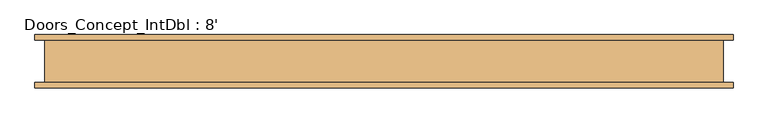
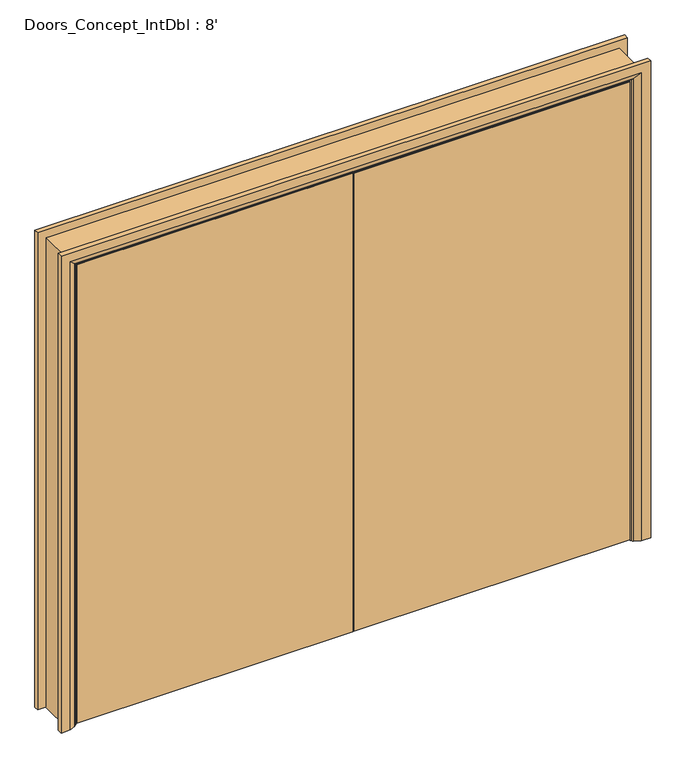
"""IFC4 building model written with IfcOpenShell, lengths in millimetres: door geometry, Doors_Concept_IntDbl : 8'."""

from ifc_helpers import new_model, si_unit, frame, origin, place, context, project, spatial, polyline, circle_curve, ellipse_curve, outline, extrude, faceted_brep, source, transform, mapped, element, save
from ifc_brep_helpers import plane_surface, cylinder_surface, advanced_brep


def doors_concept_intdbl_8_9aa9adea(model_context):
    return source(origin(), model_context, "Body", "SolidModel", [
        extrude(outline(polyline([(2110.0, -1219.2), (0.0, -1219.2), (0.0, -1179.2), (2070.0, -1179.2), (2070.0, 1179.2), (0.0, 1179.2), (0.0, 1219.2), (2110.0, 1219.2), (2110.0, -1219.2)])), frame((0.0, -76.2, 0.0), z_axis=(0.0, 1.0, 0.0), x_axis=(0.0, 0.0, 1.0)), (0.0, 0.0, 1.0), 152.4),
        faceted_brep([(-1160.2, -41.2, 0.0), (-1179.2, -41.2, 0.0), (-1179.2, -9.2, 0.0), (-1160.2, -9.2, 0.0), (-1160.2, -9.2, 2051.0), (-1160.2, -41.2, 2051.0), (-1179.2, -9.2, 2070.0), (-1179.2, -41.2, 2070.0), (1160.2, -41.2, 0.0), (1160.2, -9.2, 0.0), (1179.2, -9.2, 0.0), (1179.2, -41.2, 0.0), (1160.2, -41.2, 2051.0), (1179.2, -41.2, 2070.0), (1179.2, -9.2, 2070.0), (1160.2, -9.2, 2051.0)], [[[0, 1, 2, 3]], [[3, 4, 5, 0]], [[2, 6, 4, 3]], [[1, 7, 6, 2]], [[0, 5, 7, 1]], [[8, 9, 10, 11]], [[12, 8, 11, 13]], [[13, 11, 10, 14]], [[14, 10, 9, 15]], [[15, 9, 8, 12]], [[4, 15, 12, 5]], [[6, 14, 15, 4]], [[7, 13, 14, 6]], [[5, 12, 13, 7]]]),
        advanced_brep(
        [(1254.2, -96.2, 0.0), (1214.2, -96.2, 0.0), (1188.2, -82.2, 0.0), (1184.2, -76.2, 0.0), (1254.2, -76.2, 0.0), (1254.2, -76.2, 2145.0), (1254.2, -96.2, 2145.0), (1184.2, -76.2, 2075.0), (-1184.2, -76.2, 2075.0), (-1184.2, -76.2, 0.0), (-1254.2, -76.2, 0.0), (-1254.2, -76.2, 2145.0), (1188.2, -82.2, 2079.0), (1214.2, -96.2, 2105.0), (-1254.2, -96.2, 2145.0), (-1254.2, -96.2, 0.0), (-1214.2, -96.2, 0.0), (-1214.2, -96.2, 2105.0), (-1188.2, -82.2, 0.0), (-1188.2, -82.2, 2079.0)],
        [
            (0, 1),
            (1, 2),
            (2, 3, circle_curve(frame((1192.2, -75.2, 0.0), z_axis=(0.0, 0.0, -1.0), x_axis=(1.0, 0.0, 0.0)), 8.0622577)),
            (3, 4),
            (4, 0),
            (4, 5),
            (5, 6),
            (6, 0),
            (3, 7),
            (7, 8),
            (8, 9),
            (9, 10),
            (10, 11),
            (11, 5),
            (2, 12),
            (12, 7, ellipse_curve(frame((1192.2, -75.2, 2083.0), z_axis=(0.7071067811865475, 0.0, -0.7071067811865475), x_axis=(-0.7071067811865474, 0.0, -0.7071067811865476)), 11.4017543, 8.0622577)),
            (1, 13),
            (13, 12),
            (6, 14),
            (14, 15),
            (15, 16),
            (16, 17),
            (17, 13),
            (10, 15),
            (14, 11),
            (9, 18, circle_curve(frame((-1192.2, -75.2, 0.0), z_axis=(0.0, 0.0, -1.0), x_axis=(-1.0, 0.0, 0.0)), 8.0622577)),
            (18, 16),
            (19, 18),
            (8, 19, ellipse_curve(frame((-1192.2, -75.2, 2083.0), z_axis=(-0.7071067811865475, 0.0, -0.7071067811865475), x_axis=(-0.7071067811865474, 0.0, 0.7071067811865476)), 11.4017543, 8.0622577)),
            (19, 17),
            (12, 19),
        ],
        [
            plane_surface(frame((1184.2, -76.2, 0.0), z_axis=(0.0, 0.0, -1.0), x_axis=(0.0, 1.0, 0.0))),
            plane_surface(frame((1254.2, -96.2, 0.0), z_axis=(1.0, 0.0, 0.0), x_axis=(0.0, 0.0, 1.0))),
            plane_surface(frame((1254.2, -76.2, 0.0), z_axis=(0.0, 1.0, 0.0), x_axis=(0.0, 0.0, 1.0))),
            cylinder_surface(frame((1192.2, -75.2, 0.0), z_axis=(0.0, 0.0, -1.0), x_axis=(1.0, 0.0, 0.0)), 8.0622577),
            plane_surface(frame((1188.2, -82.2, 0.0), z_axis=(-0.4740998230350126, -0.8804710999221779, 0.0), x_axis=(0.0, 0.0, 1.0))),
            plane_surface(frame((1214.2, -96.2, 0.0), z_axis=(0.0, -1.0, 0.0), x_axis=(0.0, 0.0, 1.0))),
            plane_surface(frame((-1254.2, -96.2, 2145.0), z_axis=(-1.0, 0.0, 0.0), x_axis=(0.0, 0.0, -1.0))),
            plane_surface(frame((-1184.2, -76.2, 0.0), z_axis=(0.0, 0.0, -1.0), x_axis=(0.0, 1.0, 0.0))),
            cylinder_surface(frame((-1192.2, -75.2, 2075.0), z_axis=(0.0, 0.0, 1.0), x_axis=(-1.0, 0.0, 0.0)), 8.0622577),
            plane_surface(frame((-1188.2, -82.2, 2079.0), z_axis=(0.4740998230350183, -0.8804710999221749, 0.0), x_axis=(0.0, 0.0, -1.0))),
            plane_surface(frame((1254.2, -96.2, 2145.0), z_axis=(0.0, 0.0, 1.0), x_axis=(-1.0, 0.0, 0.0))),
            cylinder_surface(frame((1184.2, -75.2, 2083.0), z_axis=(1.0, 0.0, 0.0), x_axis=(0.0, 0.0, 1.0)), 8.0622577),
            plane_surface(frame((1188.2, -82.2, 2079.0), z_axis=(0.0, -0.8804710999221763, -0.4740998230350154), x_axis=(-1.0, 0.0, 0.0))),
        ],
        [
            (0, [[1, 2, 3, 4, 5]]),
            (1, [[6, 7, 8, -5]]),
            (2, [[9, 10, 11, 12, 13, 14, -6, -4]]),
            (3, [[15, 16, -9, -3]]),
            (4, [[17, 18, -15, -2]]),
            (5, [[-8, 19, 20, 21, 22, 23, -17, -1]]),
            (6, [[-13, 24, -20, 25]]),
            (7, [[-24, -12, 26, 27, -21]]),
            (8, [[28, -26, -11, 29]]),
            (9, [[-22, -27, -28, 30]]),
            (10, [[-14, -25, -19, -7]]),
            (11, [[31, -29, -10, -16]]),
            (12, [[-23, -30, -31, -18]]),
        ],
    ),
        advanced_brep(
        [(-1254.2, 96.2, 0.0), (-1214.2, 96.2, 0.0), (-1188.2, 82.2, 0.0), (-1184.2, 76.2, 0.0), (-1254.2, 76.2, 0.0), (-1254.2, 76.2, 2145.0), (-1254.2, 96.2, 2145.0), (-1184.2, 76.2, 2075.0), (1184.2, 76.2, 2075.0), (1184.2, 76.2, 0.0), (1254.2, 76.2, 0.0), (1254.2, 76.2, 2145.0), (-1188.2, 82.2, 2079.0), (-1214.2, 96.2, 2105.0), (1254.2, 96.2, 2145.0), (1254.2, 96.2, 0.0), (1214.2, 96.2, 0.0), (1214.2, 96.2, 2105.0), (1188.2, 82.2, 0.0), (1188.2, 82.2, 2079.0)],
        [
            (0, 1),
            (1, 2),
            (2, 3, circle_curve(frame((-1192.2, 75.2, 0.0), z_axis=(0.0, 0.0, -1.0), x_axis=(-1.0, 0.0, 0.0)), 8.0622577)),
            (3, 4),
            (4, 0),
            (4, 5),
            (5, 6),
            (6, 0),
            (3, 7),
            (7, 8),
            (8, 9),
            (9, 10),
            (10, 11),
            (11, 5),
            (2, 12),
            (12, 7, ellipse_curve(frame((-1192.2, 75.2, 2083.0), z_axis=(-0.7071067811865475, 0.0, -0.7071067811865475), x_axis=(0.7071067811865474, 0.0, -0.7071067811865476)), 11.4017543, 8.0622577)),
            (1, 13),
            (13, 12),
            (6, 14),
            (14, 15),
            (15, 16),
            (16, 17),
            (17, 13),
            (10, 15),
            (14, 11),
            (9, 18, circle_curve(frame((1192.2, 75.2, 0.0), z_axis=(0.0, 0.0, -1.0), x_axis=(1.0, 0.0, 0.0)), 8.0622577)),
            (18, 16),
            (19, 18),
            (8, 19, ellipse_curve(frame((1192.2, 75.2, 2083.0), z_axis=(0.7071067811865475, 0.0, -0.7071067811865475), x_axis=(0.7071067811865474, 0.0, 0.7071067811865476)), 11.4017543, 8.0622577)),
            (19, 17),
            (12, 19),
        ],
        [
            plane_surface(frame((-1184.2, 76.2, 0.0), z_axis=(0.0, 0.0, -1.0), x_axis=(0.0, 1.0, 0.0))),
            plane_surface(frame((-1254.2, 96.2, 0.0), z_axis=(-1.0, 0.0, 0.0), x_axis=(0.0, 0.0, 1.0))),
            plane_surface(frame((-1254.2, 76.2, 0.0), z_axis=(0.0, -1.0, 0.0), x_axis=(0.0, 0.0, 1.0))),
            cylinder_surface(frame((-1192.2, 75.2, 0.0), z_axis=(0.0, 0.0, -1.0), x_axis=(-1.0, 0.0, 0.0)), 8.0622577),
            plane_surface(frame((-1188.2, 82.2, 0.0), z_axis=(0.4740998230350183, 0.8804710999221749, 0.0), x_axis=(0.0, 0.0, 1.0))),
            plane_surface(frame((-1214.2, 96.2, 0.0), z_axis=(0.0, 1.0, 0.0), x_axis=(0.0, 0.0, 1.0))),
            plane_surface(frame((1254.2, 96.2, 2145.0), z_axis=(1.0, 0.0, 0.0), x_axis=(0.0, 0.0, -1.0))),
            plane_surface(frame((1184.2, 76.2, 0.0), z_axis=(0.0, 0.0, -1.0), x_axis=(0.0, 1.0, 0.0))),
            cylinder_surface(frame((1192.2, 75.2, 2075.0), z_axis=(0.0, 0.0, 1.0), x_axis=(1.0, 0.0, 0.0)), 8.0622577),
            plane_surface(frame((1188.2, 82.2, 2079.0), z_axis=(-0.4740998230350183, 0.8804710999221749, 0.0), x_axis=(0.0, 0.0, -1.0))),
            plane_surface(frame((-1254.2, 96.2, 2145.0), z_axis=(0.0, 0.0, 1.0), x_axis=(1.0, 0.0, 0.0))),
            cylinder_surface(frame((-1184.2, 75.2, 2083.0), z_axis=(-1.0, 0.0, 0.0), x_axis=(0.0, 0.0, 1.0)), 8.0622577),
            plane_surface(frame((-1188.2, 82.2, 2079.0), z_axis=(0.0, 0.8804710999221749, -0.4740998230350183), x_axis=(1.0, 0.0, 0.0))),
        ],
        [
            (0, [[1, 2, 3, 4, 5]]),
            (1, [[6, 7, 8, -5]]),
            (2, [[9, 10, 11, 12, 13, 14, -6, -4]]),
            (3, [[15, 16, -9, -3]]),
            (4, [[17, 18, -15, -2]]),
            (5, [[-8, 19, 20, 21, 22, 23, -17, -1]]),
            (6, [[-13, 24, -20, 25]]),
            (7, [[-24, -12, 26, 27, -21]]),
            (8, [[28, -26, -11, 29]]),
            (9, [[-22, -27, -28, 30]]),
            (10, [[-14, -25, -19, -7]]),
            (11, [[31, -29, -10, -16]]),
            (12, [[-23, -30, -31, -18]]),
        ],
    ),
        extrude(outline(polyline([(1176.2, -44.2), (1176.2, -76.2), (1.5, -76.2), (1.5, -44.2), (1176.2, -44.2)])), frame((0.0, 0.0, 5.753223), z_axis=(0.0, 0.0, 1.0), x_axis=(1.0, 0.0, 0.0)), (0.0, 0.0, 1.0), 2061.246777),
        extrude(outline(polyline([(-1.5, -44.2), (-1.5, -76.2), (-1176.2, -76.2), (-1176.2, -44.2), (-1.5, -44.2)])), frame((0.0, 0.0, 5.753223), z_axis=(0.0, 0.0, 1.0), x_axis=(1.0, 0.0, 0.0)), (0.0, 0.0, 1.0), 2061.246777),
    ])


if __name__ == "__main__":
    model = new_model("IFC4")
    model_context = context("Model", 3, world=origin())
    ifc_project = project(units=[si_unit("LENGTHUNIT", "METRE", prefix="MILLI")], contexts=[model_context])
    site = spatial("IfcSite", under=ifc_project)
    building = spatial("IfcBuilding", under=site)
    placement = place(None, origin())
    doors_concept_intdbl_8_shape = doors_concept_intdbl_8_9aa9adea(model_context)
    element("IfcDoor", 1, ObjectType="Doors_Concept_IntDbl : 8'", at=placement, inside=building, context=model_context, shape_type="MappedRepresentation", body=[
        mapped(doors_concept_intdbl_8_shape, transform((0.0, 0.0, 0.0), x_axis=(1.0, 0.0, 0.0), y_axis=(0.0, 1.0, 0.0), z_axis=(0.0, 0.0, 1.0))),
    ])
    save(model, "model.ifc")

# Revit data of these elements
# Type "Doors_Concept_IntDbl : 8'"
#   Type Mark = "53"
#   Type Comments = "Internal Double"
#   Operation = "DoubleDoorSingleSwing"
#   Construction Type Id = "GSP4R"
#   Keynote = "L10"
#   Description = "Internal Double Door"
#   Analytic Construction = "1/8 in Pilkington single glazing"
#   Visual Light Transmittance = 0.9
#   Thickness = 32 mm
#   Solar Heat Gain Coefficient = 0.78
#   Rough Width = 2438.4 mm
#   Rough Height = 2110 mm
#   Height = 2110 mm
#   Width = 2438.4 mm
#   Heat Transfer Coefficient (U) = 3.6886 W/(m²·K)
#   Define Thermal Properties by = 1
#   Function = 1
#   Material Glass = Glass
#   Material Frame = Glass, Clear Glazing
#   Material Door = Glass
#   Material Architrave = Glass
#   Wall Closure = (empty or 0)
#   Assembly Code = ""
# Element 1 (IfcDoor, "Doors_Concept_IntDbl : 8'")
#   Materials on its faces: "Glass", "Glass, Clear Glazing"
# Materials
#   "Glass": class "Glass", colour RGB 0 128 192, transparency 0.9, Description = "Soda Lime Glass", Cost = 0
#   "Glass, Clear Glazing": class "Glass", colour RGB 0 128 192, transparency 0.75, Description = "Clear glazing", Cost = 0
